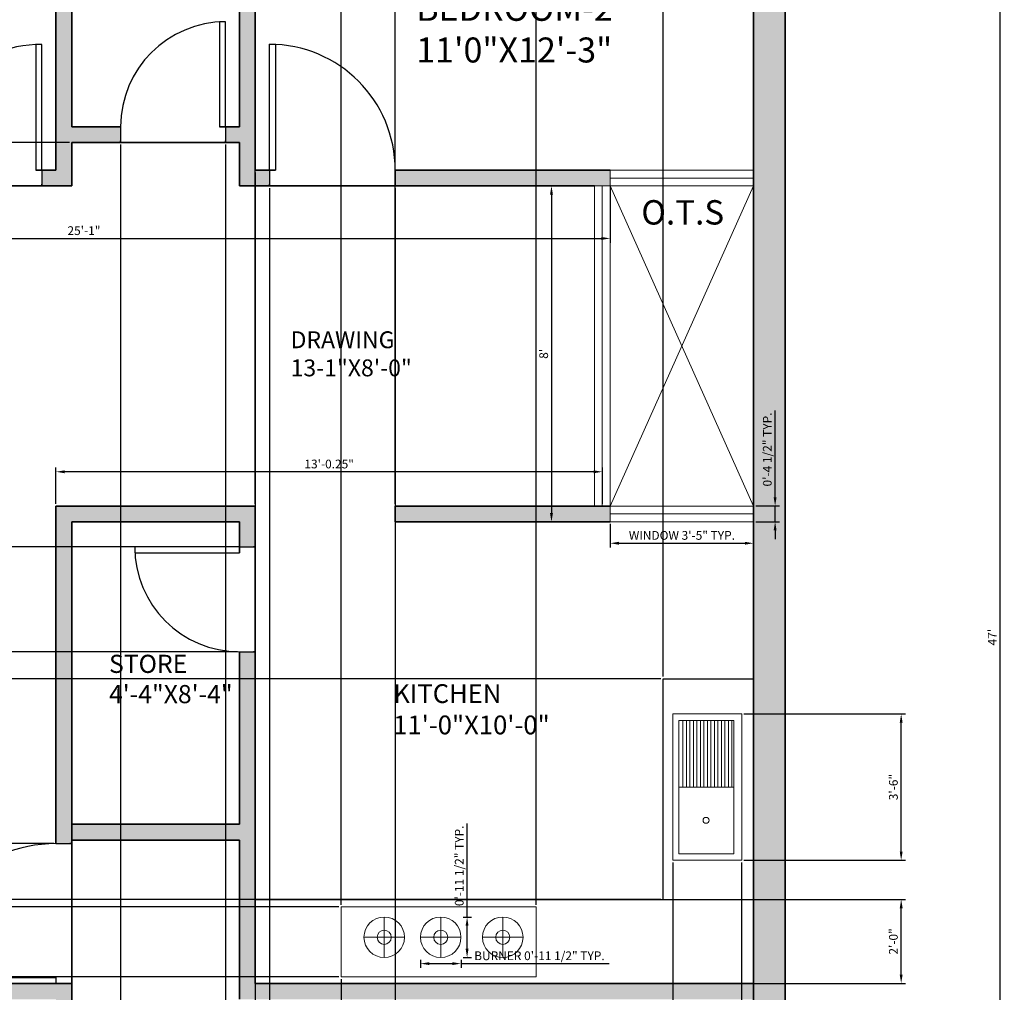
# Model space of a CAD drawing. Units: inches. Extents: x 2063 to 2524, y 2436 to 3097.
# Tile 3 of 4: x 2243 to 2524, y 2673 to 2951. Entities that reach past the tile are written whole.
import ezdxf

# ---------------------------------------------------------------- set-up
doc = ezdxf.new("R2010")
doc.units = ezdxf.units.IN
for name, color, linetype, lineweight in [('A-ANNO-DIMS', 2, 'Continuous', 18), ('A-AREA-IDEN', 7, 'Continuous', 18), ('A-DOOR', 4, 'Continuous', 25), ('A-EQPM', 8, 'Continuous', 18), ('A-FLOR-CASE', 8, 'Continuous', 25), ('A-FLOR-FIXT', 9, 'Continuous', 18), ('A-FLOR-FIXT-PATT', 9, 'Continuous', 13), ('A-FLOR-OPEN', 8, 'Continuous', 13), ('A-GLAZ', 5, 'Continuous', 18), ('A-WALL', 7, 'Continuous', 35)]:
    doc.layers.add(name, color=color, linetype=linetype, lineweight=lineweight)
doc.layers.add('A-WALL-PATT', color=251, linetype='Continuous', lineweight=13, true_color=0x636466)
doc.styles.get("Standard").update_dxf_attribs({"font": 'arial.ttf'})
doc.dimstyles.new('ISO-25', dxfattribs={"dimtxt": 2.5, "dimasz": 2.5, "dimexe": 1.25, "dimexo": 0.625, "dimtad": 1, "dimlunit": 3, "dimtxsty": 'Standard', "dimcen": 2.5, "dimadec": 0, "dimazin": 0, "dimtfac": 1, "dimtmove": 0, "dimatfit": 3, "dimfxl": 1, "dimarcsym": 0})

# ---------------------------------------------------------------- blocks, each defined once
blk = doc.blocks.new('*U3')
for p, q in [((0, 0), (0, -4)), ((-36, 0), (-36, -4))]:
    blk.add_line(p, q)
blk.add_lwpolyline([(0, 0), (0, 36), (-1.75, 36), (-1.75, 0)], close=True)
blk.add_arc((0, 0), 36, 90, 180)
blk = doc.blocks.new('*U4')
for p, q in [((-30, 0), (-30, -4)), ((0, 0), (0, -4))]:
    blk.add_line(p, q)
blk.add_lwpolyline([(0, 0), (0, 30), (-1.75, 30), (-1.75, 0)], close=True)
blk.add_arc((0, 0), 30, 90, 180)
blk = doc.blocks.new('*U2')
for p, q in [((0, 0), (0, -4)), ((36, 0), (36, -4))]:
    blk.add_line(p, q)
blk.add_lwpolyline([(0, 0), (0, 36), (1.75, 36), (1.75, 0)], close=True)
blk.add_arc((0, 0), 36, 0, 90)
blk = doc.blocks.new('*U6')
for p, q in [((-30, 0), (-30, -4)), ((0, 0), (0, -4))]:
    blk.add_line(p, q)
blk.add_lwpolyline([(0, 0), (0, 30), (-1.75, 30), (-1.75, 0)], close=True)
blk.add_arc((0, 0), 30, 90, 180)
blk = doc.blocks.new('*U5')
for p, q in [((0, 0), (0, -4)), ((40, 0), (40, -4))]:
    blk.add_line(p, q)
blk.add_lwpolyline([(0, 0), (0, 40), (1.75, 40), (1.75, 0)], close=True)
blk.add_arc((0, 0), 40, 0, 90)
blk = doc.blocks.new('*D11')
at = {"layer": 'A-ANNO-DIMS', "color": 0, "lineweight": -2, "transparency": 16777216}
for p, q in [((2110.76, 2902.49), (2110.76, 2886.87)), ((2411.76, 2902.49), (2411.76, 2886.87)), ((2113.26, 2888.12), (2409.26, 2888.12))]:
    blk.add_line(p, q, dxfattribs=at)
at = {"layer": 'A-ANNO-DIMS', "color": 0, "transparency": 16777216}
for points in [[(2113.26, 2888.53), (2113.26, 2887.7), (2110.76, 2888.12)], [(2409.26, 2888.53), (2409.26, 2887.7), (2411.76, 2888.12)]]:
    blk.add_solid(points, dxfattribs=at)
at = {"layer": 'Defpoints', "color": 0, "transparency": 16777216}
for p in [(2110.76, 2903.12), (2411.76, 2903.12), (2411.76, 2888.12)]:
    blk.add_point(p, dxfattribs=at)
at = {"layer": 'A-ANNO-DIMS', "color": 0, "transparency": 16777216, "insert": (2261.26, 2890.02), "char_height": 2.5, "attachment_point": 5}
blk.add_mtext('25\'-1"', dxfattribs=at)
blk = doc.blocks.new('*D12')
at = {"layer": 'A-ANNO-DIMS', "color": 0, "lineweight": -2, "transparency": 16777216}
for p, q in [((2406.64, 2903.12), (2393.71, 2903.12)), ((2394.96, 2900.62), (2394.96, 2809.62)), ((2406.64, 2807.12), (2393.71, 2807.12))]:
    blk.add_line(p, q, dxfattribs=at)
at = {"layer": 'A-ANNO-DIMS', "color": 0, "transparency": 16777216}
for points in [[(2394.54, 2900.62), (2395.38, 2900.62), (2394.96, 2903.12)], [(2394.54, 2809.62), (2395.38, 2809.62), (2394.96, 2807.12)]]:
    blk.add_solid(points, dxfattribs=at)
at = {"layer": 'Defpoints', "color": 0, "transparency": 16777216}
for p in [(2407.26, 2903.12), (2394.96, 2807.12), (2407.26, 2807.12)]:
    blk.add_point(p, dxfattribs=at)
at = {"layer": 'A-ANNO-DIMS', "color": 0, "transparency": 16777216, "insert": (2393.06, 2855.12), "char_height": 2.5, "attachment_point": 5, "rotation": 90}
blk.add_mtext("8'", dxfattribs=at)
blk = doc.blocks.new('*D13')
at = {"layer": 'A-ANNO-DIMS', "color": 0, "lineweight": -2, "transparency": 16777216}
for p, q in [((2253.26, 2812.24), (2253.26, 2822.65)), ((2407.01, 2821.4), (2255.76, 2821.4)), ((2409.51, 2812.24), (2409.51, 2822.65))]:
    blk.add_line(p, q, dxfattribs=at)
at = {"layer": 'A-ANNO-DIMS', "color": 0, "transparency": 16777216}
for points in [[(2255.76, 2821.81), (2255.76, 2820.98), (2253.26, 2821.4)], [(2407.01, 2821.81), (2407.01, 2820.98), (2409.51, 2821.4)]]:
    blk.add_solid(points, dxfattribs=at)
at = {"layer": 'Defpoints', "color": 0, "transparency": 16777216}
for p in [(2253.26, 2821.4), (2253.26, 2811.62), (2409.51, 2811.62)]:
    blk.add_point(p, dxfattribs=at)
at = {"layer": 'A-ANNO-DIMS', "color": 0, "transparency": 16777216, "insert": (2331.39, 2823.3), "char_height": 2.5, "attachment_point": 5}
blk.add_mtext('13\'-0.25"', dxfattribs=at)
blk = doc.blocks.new('*D15')
at = {"layer": 'A-ANNO-DIMS', "color": 0, "lineweight": -2, "transparency": 16777216}
for p, q in [((2462.39, 3056.12), (2524.46, 3056.12)), ((2523.21, 3053.62), (2523.21, 2494.62)), ((2462.39, 2492.12), (2524.46, 2492.12))]:
    blk.add_line(p, q, dxfattribs=at)
at = {"layer": 'A-ANNO-DIMS', "color": 0, "transparency": 16777216}
for points in [[(2522.79, 3053.62), (2523.62, 3053.62), (2523.21, 3056.12)], [(2522.79, 2494.62), (2523.62, 2494.62), (2523.21, 2492.12)]]:
    blk.add_solid(points, dxfattribs=at)
at = {"layer": 'Defpoints', "color": 0, "transparency": 16777216}
for p in [(2461.76, 3056.12), (2461.76, 2492.12), (2523.21, 2492.12)]:
    blk.add_point(p, dxfattribs=at)
at = {"layer": 'A-ANNO-DIMS', "color": 0, "transparency": 16777216, "insert": (2521.33, 2774.12), "char_height": 2.5, "attachment_point": 5, "rotation": 90}
blk.add_mtext("47'", dxfattribs=at)
blk = doc.blocks.new('COOKTOP-BURNER')
for p, q in [((5.79, 11.58), (5.79, 0)), ((5.79, 5.79), (0, 5.79)), ((5.79, 0), (5.79, 5.79)), ((5.79, 5.79), (11.58, 5.79)), ((11.58, 5.79), (5.79, 5.79))]:
    blk.add_line(p, q)
for radius in [5.79, 2.02]:
    blk.add_circle((5.79, 5.79), radius)
blk = doc.blocks.new('WIN-OTS-41IN')
for p, q in [((0, 4.5), (41, 4.5)), ((0, 2.25), (41, 2.25)), ((0, 0), (41, 0))]:
    blk.add_line(p, q)
blk = doc.blocks.new('*D22')
at = {"layer": 'A-ANNO-DIMS', "color": 0, "lineweight": -2, "transparency": 16777216}
for p, q in [((2357.51, 2681.89), (2357.51, 2679.53)), ((2360.01, 2680.78), (2366.59, 2680.78)), ((2369.09, 2681.89), (2369.09, 2679.53)), ((2369.09, 2680.78), (2411.45, 2680.78))]:
    blk.add_line(p, q, dxfattribs=at)
at = {"layer": 'A-ANNO-DIMS', "color": 0, "transparency": 16777216}
for points in [[(2360.01, 2681.2), (2360.01, 2680.37), (2357.51, 2680.78)], [(2366.59, 2681.2), (2366.59, 2680.37), (2369.09, 2680.78)]]:
    blk.add_solid(points, dxfattribs=at)
at = {"layer": 'Defpoints', "color": 0, "transparency": 16777216}
for p in [(2357.51, 2682.52), (2369.09, 2682.52), (2369.09, 2680.78)]:
    blk.add_point(p, dxfattribs=at)
at = {"layer": 'A-ANNO-DIMS', "color": 0, "transparency": 16777216, "insert": (2391.52, 2682.7), "char_height": 2.5, "attachment_point": 5}
blk.add_mtext('BURNER 0\'-11 1/2" TYP.', dxfattribs=at)
blk = doc.blocks.new('*D23')
at = {"layer": 'A-ANNO-DIMS', "color": 0, "lineweight": -2, "transparency": 16777216}
for p, q in [((2370.83, 2694.1), (2370.83, 2720.86)), ((2369.71, 2694.1), (2372.08, 2694.1)), ((2370.83, 2685.02), (2370.83, 2691.6)), ((2369.71, 2682.52), (2372.08, 2682.52))]:
    blk.add_line(p, q, dxfattribs=at)
at = {"layer": 'A-ANNO-DIMS', "color": 0, "transparency": 16777216}
for points in [[(2370.41, 2691.6), (2371.24, 2691.6), (2370.83, 2694.1)], [(2370.41, 2685.02), (2371.24, 2685.02), (2370.83, 2682.52)]]:
    blk.add_solid(points, dxfattribs=at)
at = {"layer": 'Defpoints', "color": 0, "transparency": 16777216}
for p in [(2369.09, 2694.1), (2370.83, 2694.1), (2369.09, 2682.52)]:
    blk.add_point(p, dxfattribs=at)
at = {"layer": 'A-ANNO-DIMS', "color": 0, "transparency": 16777216, "insert": (2368.91, 2708.73), "char_height": 2.5, "attachment_point": 5, "rotation": 90}
blk.add_mtext('0\'-11 1/2" TYP.', dxfattribs=at)
blk = doc.blocks.new('*D26')
at = {"layer": 'A-ANNO-DIMS', "color": 0, "lineweight": -2, "transparency": 16777216}
for p, q in [((2411.76, 2806.49), (2411.76, 2799.72)), ((2452.76, 2806.49), (2452.76, 2799.72)), ((2414.26, 2800.97), (2450.26, 2800.97))]:
    blk.add_line(p, q, dxfattribs=at)
at = {"layer": 'A-ANNO-DIMS', "color": 0, "transparency": 16777216}
for points in [[(2414.26, 2801.38), (2414.26, 2800.55), (2411.76, 2800.97)], [(2450.26, 2801.38), (2450.26, 2800.55), (2452.76, 2800.97)]]:
    blk.add_solid(points, dxfattribs=at)
at = {"layer": 'Defpoints', "color": 0, "transparency": 16777216}
for p in [(2411.76, 2807.12), (2452.76, 2807.12), (2452.76, 2800.97)]:
    blk.add_point(p, dxfattribs=at)
at = {"layer": 'A-ANNO-DIMS', "color": 0, "transparency": 16777216, "insert": (2432.26, 2802.89), "char_height": 2.5, "attachment_point": 5}
blk.add_mtext('WINDOW 3\'-5" TYP.', dxfattribs=at)
blk = doc.blocks.new('*D27')
at = {"layer": 'A-ANNO-DIMS', "color": 0, "lineweight": -2, "transparency": 16777216}
for p, q in [((2458.91, 2814.12), (2458.91, 2838.93)), ((2453.39, 2811.62), (2460.16, 2811.62)), ((2458.91, 2807.12), (2458.91, 2811.62)), ((2453.39, 2807.12), (2460.16, 2807.12)), ((2458.91, 2804.62), (2458.91, 2802.12))]:
    blk.add_line(p, q, dxfattribs=at)
at = {"layer": 'A-ANNO-DIMS', "color": 0, "transparency": 16777216}
for points in [[(2458.5, 2814.12), (2459.33, 2814.12), (2458.91, 2811.62)], [(2458.5, 2804.62), (2459.33, 2804.62), (2458.91, 2807.12)]]:
    blk.add_solid(points, dxfattribs=at)
at = {"layer": 'Defpoints', "color": 0, "transparency": 16777216}
for p in [(2452.76, 2811.62), (2458.91, 2811.62), (2452.76, 2807.12)]:
    blk.add_point(p, dxfattribs=at)
at = {"layer": 'A-ANNO-DIMS', "color": 0, "transparency": 16777216, "insert": (2457, 2827.77), "char_height": 2.5, "attachment_point": 5, "rotation": 90}
blk.add_mtext('0\'-4 1/2" TYP.', dxfattribs=at)
blk = doc.blocks.new('*D34')
at = {"layer": 'A-ANNO-DIMS', "color": 0, "lineweight": -2, "transparency": 16777216}
for p, q in [((2271.76, 2914.94), (2271.76, 2457.67)), ((2301.76, 2914.94), (2301.76, 2457.67)), ((2274.26, 2458.92), (2299.26, 2458.92))]:
    blk.add_line(p, q, dxfattribs=at)
at = {"layer": 'A-ANNO-DIMS', "color": 0, "transparency": 16777216}
for points in [[(2274.26, 2459.33), (2274.26, 2458.5), (2271.76, 2458.92)], [(2299.26, 2459.33), (2299.26, 2458.5), (2301.76, 2458.92)]]:
    blk.add_solid(points, dxfattribs=at)
at = {"layer": 'Defpoints', "color": 0, "transparency": 16777216}
for p in [(2271.76, 2915.57), (2301.76, 2915.57), (2301.76, 2458.92)]:
    blk.add_point(p, dxfattribs=at)
at = {"layer": 'A-ANNO-DIMS', "color": 0, "transparency": 16777216, "insert": (2286.76, 2460.82), "char_height": 2.5, "attachment_point": 5}
blk.add_mtext('2\'-6"', dxfattribs=at)
blk = doc.blocks.new('*D35')
at = {"layer": 'A-ANNO-DIMS', "color": 0, "lineweight": -2, "transparency": 16777216}
for p, q in [((2068.56, 2915.57), (2068.56, 2931.55)), ((2257.14, 2915.57), (2067.31, 2915.57)), ((2068.56, 2905.62), (2068.56, 2913.07)), ((2257.14, 2903.12), (2067.31, 2903.12))]:
    blk.add_line(p, q, dxfattribs=at)
at = {"layer": 'A-ANNO-DIMS', "color": 0, "transparency": 16777216}
for points in [[(2068.15, 2913.07), (2068.98, 2913.07), (2068.56, 2915.57)], [(2068.15, 2905.62), (2068.98, 2905.62), (2068.56, 2903.12)]]:
    blk.add_solid(points, dxfattribs=at)
at = {"layer": 'Defpoints', "color": 0, "transparency": 16777216}
for p in [(2068.56, 2915.57), (2257.76, 2915.57), (2257.76, 2903.12)]:
    blk.add_point(p, dxfattribs=at)
at = {"layer": 'A-ANNO-DIMS', "color": 0, "transparency": 16777216, "insert": (2066.65, 2924.81), "char_height": 2.5, "attachment_point": 5, "rotation": 90}
blk.add_mtext('1\'-0 1/2"', dxfattribs=at)
blk = doc.blocks.new('*D36')
at = {"layer": 'A-ANNO-DIMS', "color": 0, "lineweight": -2, "transparency": 16777216}
for p, q in [((2314.3, 2902.49), (2314.3, 2457.67)), ((2350.3, 2902.49), (2350.3, 2457.67)), ((2316.8, 2458.92), (2347.8, 2458.92))]:
    blk.add_line(p, q, dxfattribs=at)
at = {"layer": 'A-ANNO-DIMS', "color": 0, "transparency": 16777216}
for points in [[(2316.8, 2459.33), (2316.8, 2458.5), (2314.3, 2458.92)], [(2347.8, 2459.33), (2347.8, 2458.5), (2350.3, 2458.92)]]:
    blk.add_solid(points, dxfattribs=at)
at = {"layer": 'Defpoints', "color": 0, "transparency": 16777216}
for p in [(2314.3, 2903.12), (2350.3, 2903.12), (2350.3, 2458.92)]:
    blk.add_point(p, dxfattribs=at)
at = {"layer": 'A-ANNO-DIMS', "color": 0, "transparency": 16777216, "insert": (2332.3, 2460.82), "char_height": 2.5, "attachment_point": 5}
blk.add_mtext('3\'-0"', dxfattribs=at)
blk = doc.blocks.new('*D38')
at = {"layer": 'A-ANNO-DIMS', "color": 0, "lineweight": -2, "transparency": 16777216}
for p, q in [((2310.26, 2812.24), (2310.26, 3090.57)), ((2312.76, 3089.32), (2347.8, 3089.32)), ((2350.3, 2812.24), (2350.3, 3090.57))]:
    blk.add_line(p, q, dxfattribs=at)
at = {"layer": 'A-ANNO-DIMS', "color": 0, "transparency": 16777216}
for points in [[(2312.76, 3089.73), (2312.76, 3088.9), (2310.26, 3089.32)], [(2347.8, 3089.73), (2347.8, 3088.9), (2350.3, 3089.32)]]:
    blk.add_solid(points, dxfattribs=at)
at = {"layer": 'Defpoints', "color": 0, "transparency": 16777216}
for p in [(2350.3, 3089.32), (2310.26, 2811.62), (2350.3, 2811.62)]:
    blk.add_point(p, dxfattribs=at)
at = {"layer": 'A-ANNO-DIMS', "color": 0, "transparency": 16777216, "insert": (2330.28, 3091.22), "char_height": 2.5, "attachment_point": 5}
blk.add_mtext('3\'-4"', dxfattribs=at)
blk = doc.blocks.new('*D39')
at = {"layer": 'A-ANNO-DIMS', "color": 0, "lineweight": -2, "transparency": 16777216}
for p, q in [((2426.9, 2762.84), (2426.9, 3090.57)), ((2429.4, 3089.32), (2450.26, 3089.32)), ((2452.76, 2762.84), (2452.76, 3090.57))]:
    blk.add_line(p, q, dxfattribs=at)
at = {"layer": 'A-ANNO-DIMS', "color": 0, "transparency": 16777216}
for points in [[(2429.4, 3089.73), (2429.4, 3088.9), (2426.9, 3089.32)], [(2450.26, 3089.73), (2450.26, 3088.9), (2452.76, 3089.32)]]:
    blk.add_solid(points, dxfattribs=at)
at = {"layer": 'Defpoints', "color": 0, "transparency": 16777216}
for p in [(2452.76, 3089.32), (2426.9, 2762.21), (2452.76, 2762.21)]:
    blk.add_point(p, dxfattribs=at)
at = {"layer": 'A-ANNO-DIMS', "color": 0, "transparency": 16777216, "insert": (2439.83, 3091.2), "char_height": 2.5, "attachment_point": 5}
blk.add_mtext('2\'-2"', dxfattribs=at)
blk = doc.blocks.new('*D40')
at = {"layer": 'A-ANNO-DIMS', "color": 0, "lineweight": -2, "transparency": 16777216}
for p, q in [((2310.89, 2699.12), (2496.21, 2699.12)), ((2494.96, 2677.62), (2494.96, 2696.62)), ((2310.89, 2675.12), (2496.21, 2675.12))]:
    blk.add_line(p, q, dxfattribs=at)
at = {"layer": 'A-ANNO-DIMS', "color": 0, "transparency": 16777216}
for points in [[(2494.55, 2696.62), (2495.38, 2696.62), (2494.96, 2699.12)], [(2494.55, 2677.62), (2495.38, 2677.62), (2494.96, 2675.12)]]:
    blk.add_solid(points, dxfattribs=at)
at = {"layer": 'Defpoints', "color": 0, "transparency": 16777216}
for p in [(2310.26, 2699.12), (2494.96, 2699.12), (2310.26, 2675.12)]:
    blk.add_point(p, dxfattribs=at)
at = {"layer": 'A-ANNO-DIMS', "color": 0, "transparency": 16777216, "insert": (2493.06, 2687.12), "char_height": 2.5, "attachment_point": 5, "rotation": 90}
blk.add_mtext('2\'-0"', dxfattribs=at)
blk = doc.blocks.new('*D41')
at = {"layer": 'A-ANNO-DIMS', "color": 0, "lineweight": -2, "transparency": 16777216}
for p, q in [((2305.15, 2799.95), (2067.31, 2799.95)), ((2068.56, 2772.45), (2068.56, 2797.45)), ((2305.14, 2769.95), (2067.31, 2769.95))]:
    blk.add_line(p, q, dxfattribs=at)
at = {"layer": 'A-ANNO-DIMS', "color": 0, "transparency": 16777216}
for points in [[(2068.15, 2797.45), (2068.98, 2797.45), (2068.56, 2799.95)], [(2068.15, 2772.45), (2068.98, 2772.45), (2068.56, 2769.95)]]:
    blk.add_solid(points, dxfattribs=at)
at = {"layer": 'Defpoints', "color": 0, "transparency": 16777216}
for p in [(2068.56, 2799.95), (2305.78, 2799.95), (2305.76, 2769.95)]:
    blk.add_point(p, dxfattribs=at)
at = {"layer": 'A-ANNO-DIMS', "color": 0, "transparency": 16777216, "insert": (2066.66, 2784.95), "char_height": 2.5, "attachment_point": 5, "rotation": 90}
blk.add_mtext('2\'-6"', dxfattribs=at)
blk = doc.blocks.new('*D42')
at = {"layer": 'A-ANNO-DIMS', "color": 0, "lineweight": -2, "transparency": 16777216}
for p, q in [((2426.27, 2762.21), (2067.31, 2762.21)), ((2068.56, 2701.62), (2068.56, 2759.71)), ((2426.27, 2699.12), (2067.31, 2699.12))]:
    blk.add_line(p, q, dxfattribs=at)
at = {"layer": 'A-ANNO-DIMS', "color": 0, "transparency": 16777216}
for points in [[(2068.15, 2759.71), (2068.98, 2759.71), (2068.56, 2762.21)], [(2068.15, 2701.62), (2068.98, 2701.62), (2068.56, 2699.12)]]:
    blk.add_solid(points, dxfattribs=at)
at = {"layer": 'Defpoints', "color": 0, "transparency": 16777216}
for p in [(2068.56, 2762.21), (2426.9, 2762.21), (2426.9, 2699.12)]:
    blk.add_point(p, dxfattribs=at)
at = {"layer": 'A-ANNO-DIMS', "color": 0, "transparency": 16777216, "insert": (2066.66, 2730.67), "char_height": 2.5, "attachment_point": 5, "rotation": 90}
blk.add_mtext('5\'-3"', dxfattribs=at)
blk = doc.blocks.new('*D43')
at = {"layer": 'A-ANNO-DIMS', "color": 0, "lineweight": -2, "transparency": 16777216}
for p, q in [((2429.67, 2709.7), (2429.67, 2457.67)), ((2449.35, 2709.7), (2449.35, 2457.67)), ((2432.17, 2458.92), (2446.85, 2458.92))]:
    blk.add_line(p, q, dxfattribs=at)
at = {"layer": 'A-ANNO-DIMS', "color": 0, "transparency": 16777216}
for points in [[(2432.17, 2459.33), (2432.17, 2458.5), (2429.67, 2458.92)], [(2446.85, 2459.33), (2446.85, 2458.5), (2449.35, 2458.92)]]:
    blk.add_solid(points, dxfattribs=at)
at = {"layer": 'Defpoints', "color": 0, "transparency": 16777216}
for p in [(2429.67, 2710.33), (2449.35, 2710.33), (2449.35, 2458.92)]:
    blk.add_point(p, dxfattribs=at)
at = {"layer": 'A-ANNO-DIMS', "color": 0, "transparency": 16777216, "insert": (2439.51, 2460.84), "char_height": 2.5, "attachment_point": 5}
blk.add_mtext('1\'-7 1/2"', dxfattribs=at)
blk = doc.blocks.new('*D44')
at = {"layer": 'A-ANNO-DIMS', "color": 0, "lineweight": -2, "transparency": 16777216}
for p, q in [((2449.98, 2752.17), (2496.21, 2752.17)), ((2494.96, 2712.83), (2494.96, 2749.67)), ((2449.98, 2710.33), (2496.21, 2710.33))]:
    blk.add_line(p, q, dxfattribs=at)
at = {"layer": 'A-ANNO-DIMS', "color": 0, "transparency": 16777216}
for points in [[(2494.55, 2749.67), (2495.38, 2749.67), (2494.96, 2752.17)], [(2494.55, 2712.83), (2495.38, 2712.83), (2494.96, 2710.33)]]:
    blk.add_solid(points, dxfattribs=at)
at = {"layer": 'Defpoints', "color": 0, "transparency": 16777216}
for p in [(2449.35, 2752.17), (2494.96, 2752.17), (2449.35, 2710.33)]:
    blk.add_point(p, dxfattribs=at)
at = {"layer": 'A-ANNO-DIMS', "color": 0, "transparency": 16777216, "insert": (2493.06, 2731.25), "char_height": 2.5, "attachment_point": 5, "rotation": 90}
blk.add_mtext('3\'-6"', dxfattribs=at)
blk = doc.blocks.new('*D45')
at = {"layer": 'A-ANNO-DIMS', "color": 0, "lineweight": -2, "transparency": 16777216}
for p, q in [((2252.63, 2715.09), (2067.31, 2715.09)), ((2068.56, 2677.62), (2068.56, 2712.59)), ((2252.64, 2675.12), (2067.31, 2675.12))]:
    blk.add_line(p, q, dxfattribs=at)
at = {"layer": 'A-ANNO-DIMS', "color": 0, "transparency": 16777216}
for points in [[(2068.15, 2712.59), (2068.98, 2712.59), (2068.56, 2715.09)], [(2068.15, 2677.62), (2068.98, 2677.62), (2068.56, 2675.12)]]:
    blk.add_solid(points, dxfattribs=at)
at = {"layer": 'Defpoints', "color": 0, "transparency": 16777216}
for p in [(2068.56, 2715.09), (2253.26, 2715.09), (2253.26, 2675.12)]:
    blk.add_point(p, dxfattribs=at)
at = {"layer": 'A-ANNO-DIMS', "color": 0, "transparency": 16777216, "insert": (2066.66, 2695.1), "char_height": 2.5, "attachment_point": 5, "rotation": 90}
blk.add_mtext('3\'-4"', dxfattribs=at)
blk = doc.blocks.new('*D48')
at = {"layer": 'A-ANNO-DIMS', "color": 0, "lineweight": -2, "transparency": 16777216}
for p, q in [((2310.26, 2906.99), (2310.26, 2457.67)), ((2314.3, 2902.49), (2314.3, 2457.67)), ((2307.76, 2458.92), (2305.26, 2458.92)), ((2310.26, 2458.92), (2314.3, 2458.92)), ((2316.8, 2458.92), (2327.2, 2458.92))]:
    blk.add_line(p, q, dxfattribs=at)
at = {"layer": 'A-ANNO-DIMS', "color": 0, "transparency": 16777216}
for points in [[(2307.76, 2459.33), (2307.76, 2458.5), (2310.26, 2458.92)], [(2316.8, 2459.33), (2316.8, 2458.5), (2314.3, 2458.92)]]:
    blk.add_solid(points, dxfattribs=at)
at = {"layer": 'Defpoints', "color": 0, "transparency": 16777216}
for p in [(2310.26, 2907.62), (2314.3, 2903.12), (2314.3, 2458.92)]:
    blk.add_point(p, dxfattribs=at)
at = {"layer": 'A-ANNO-DIMS', "color": 0, "transparency": 16777216, "insert": (2323.25, 2460.82), "char_height": 2.5, "attachment_point": 5}
blk.add_mtext('0\'-4"', dxfattribs=at)
blk = doc.blocks.new('*D49')
at = {"layer": 'A-ANNO-DIMS', "color": 0, "lineweight": -2, "transparency": 16777216}
for p, q in [((2334.8, 2697.62), (2334.8, 3090.57)), ((2337.3, 3089.32), (2388.07, 3089.32)), ((2390.57, 2697.62), (2390.57, 3090.57))]:
    blk.add_line(p, q, dxfattribs=at)
at = {"layer": 'A-ANNO-DIMS', "color": 0, "transparency": 16777216}
for points in [[(2337.3, 3089.73), (2337.3, 3088.9), (2334.8, 3089.32)], [(2388.07, 3089.73), (2388.07, 3088.9), (2390.57, 3089.32)]]:
    blk.add_solid(points, dxfattribs=at)
at = {"layer": 'Defpoints', "color": 0, "transparency": 16777216}
for p in [(2390.57, 3089.32), (2334.8, 2696.99), (2390.57, 2696.99)]:
    blk.add_point(p, dxfattribs=at)
at = {"layer": 'A-ANNO-DIMS', "color": 0, "transparency": 16777216, "insert": (2362.68, 3091.22), "char_height": 2.5, "attachment_point": 5}
blk.add_mtext('4\'-8"', dxfattribs=at)
blk = doc.blocks.new('*D50')
at = {"layer": 'A-ANNO-DIMS', "color": 0, "lineweight": -2, "transparency": 16777216}
for p, q in [((2334.17, 2696.99), (2067.31, 2696.99)), ((2068.56, 2679.49), (2068.56, 2694.49)), ((2334.17, 2676.99), (2067.31, 2676.99))]:
    blk.add_line(p, q, dxfattribs=at)
at = {"layer": 'A-ANNO-DIMS', "color": 0, "transparency": 16777216}
for points in [[(2068.15, 2694.49), (2068.98, 2694.49), (2068.56, 2696.99)], [(2068.15, 2679.49), (2068.98, 2679.49), (2068.56, 2676.99)]]:
    blk.add_solid(points, dxfattribs=at)
at = {"layer": 'Defpoints', "color": 0, "transparency": 16777216}
for p in [(2068.56, 2696.99), (2334.8, 2696.99), (2334.8, 2676.99)]:
    blk.add_point(p, dxfattribs=at)
at = {"layer": 'A-ANNO-DIMS', "color": 0, "transparency": 16777216, "insert": (2066.66, 2686.99), "char_height": 2.5, "attachment_point": 5, "rotation": 90}
blk.add_mtext('1\'-8"', dxfattribs=at)
blk = doc.blocks.new('*D51')
at = {"layer": 'A-ANNO-DIMS', "color": 0, "lineweight": -2, "transparency": 16777216}
for p, q in [((2334.8, 2676.36), (2334.8, 2457.67)), ((2310.26, 2674.49), (2310.26, 2457.67)), ((2312.76, 2458.92), (2332.3, 2458.92))]:
    blk.add_line(p, q, dxfattribs=at)
at = {"layer": 'A-ANNO-DIMS', "color": 0, "transparency": 16777216}
for points in [[(2312.76, 2459.33), (2312.76, 2458.5), (2310.26, 2458.92)], [(2332.3, 2459.33), (2332.3, 2458.5), (2334.8, 2458.92)]]:
    blk.add_solid(points, dxfattribs=at)
at = {"layer": 'Defpoints', "color": 0, "transparency": 16777216}
for p in [(2310.26, 2675.12), (2334.8, 2676.99), (2334.8, 2458.92)]:
    blk.add_point(p, dxfattribs=at)
at = {"layer": 'A-ANNO-DIMS', "color": 0, "transparency": 16777216, "insert": (2322.53, 2460.84), "char_height": 2.5, "attachment_point": 5}
blk.add_mtext('2\'-0 1/2"', dxfattribs=at)

msp = doc.modelspace()

# ---------------------------------------------------------------- hatches: boundary and pattern name
at = {"layer": 'A-FLOR-FIXT-PATT'}
h = msp.add_hatch(dxfattribs=at)
h.set_pattern_fill('ANSI31', color=256, scale=0.3149013, angle=45, style=0)
h.paths.add_polyline_path([(2432.04, 2731.223), (2447.04, 2731.223), (2447.04, 2750.267), (2432.04, 2750.267)])
at = {"layer": 'A-WALL-PATT'}
h = msp.add_hatch(color=256, dxfattribs=at)
h.dxf.hatch_style = 1
h.paths.add_polyline_path([(2110.763, 2670.618), (2110.763, 2676.643), (2110.763, 3047.118), (2452.763, 3047.118), (2452.763, 2501.118), (2200.478, 2501.118), (2200.478, 2492.118), (2461.763, 2492.118), (2461.763, 3056.118), (2101.763, 3056.118), (2101.763, 2492.118), (2149.478, 2492.118), (2149.478, 2496.618), (2149.478, 2501.118), (2110.763, 2501.118)])
h.paths.add_polyline_path([(2257.763, 2675.118), (2257.255, 2675.091), (2253.255, 2675.091), (2213.255, 2675.091), (2151.474, 2675.107), (2151.474, 2674.543), (2151.474, 2670.618), (2253.263, 2670.618), (2253.263, 2501.118), (2257.763, 2501.118)], flags=17)
h.paths.add_polyline_path([(2310.263, 3006.972), (2305.763, 3006.972), (2305.763, 2920.067), (2301.763, 2920.067), (2301.759, 2920.067), (2301.759, 2920.063), (2301.759, 2916.063), (2301.759, 2915.567), (2305.763, 2915.567), (2305.763, 2903.118), (2314.3, 2903.118), (2314.3, 2903.618), (2314.3, 2907.618), (2310.263, 2907.618)], flags=17)
h.paths.add_polyline_path([(2257.763, 3006.972), (2253.263, 3006.972), (2253.263, 2907.618), (2249.263, 2907.618), (2249.258, 2907.618), (2249.258, 2907.597), (2249.258, 2903.597), (2249.258, 2903.118), (2257.763, 2903.118), (2257.763, 2915.567), (2271.759, 2915.567), (2271.759, 2916.063), (2271.759, 2920.067), (2257.763, 2920.067)], flags=17)
h.paths.add_polyline_path([(2213.258, 2907.618), (2110.763, 2907.618), (2110.763, 2903.118), (2213.258, 2903.118), (2213.258, 2903.597)], flags=17)
h.paths.add_polyline_path([(2411.763, 2907.618), (2350.3, 2907.618), (2350.3, 2903.618), (2350.3, 2903.118), (2407.264, 2903.118), (2411.763, 2903.118)], flags=17)
h.paths.add_polyline_path([(2260.327, 2964.034), (2307.905, 2964.034), (2307.905, 2989.359), (2260.327, 2989.359)], flags=25)
h = msp.add_hatch(color=256, dxfattribs=at)
h.dxf.hatch_style = 1
h.paths.add_polyline_path([(2310.263, 2811.618), (2305.763, 2811.618), (2253.263, 2811.618), (2253.263, 2716.118), (2253.255, 2715.091), (2257.255, 2715.091), (2257.763, 2715.091), (2257.763, 2720.618), (2257.763, 2807.118), (2305.763, 2807.118), (2305.763, 2799.95), (2305.776, 2799.95), (2309.776, 2799.95), (2310.263, 2799.95)])
h.paths.add_polyline_path([(2310.263, 2769.95), (2309.776, 2769.95), (2305.763, 2769.95), (2305.763, 2720.618), (2257.763, 2720.618), (2257.763, 2716.118), (2305.763, 2716.118), (2305.763, 2670.618), (2310.263, 2670.618), (2452.763, 2670.618), (2452.763, 2675.118), (2426.899, 2675.118), (2310.263, 2675.118)])
h = msp.add_hatch(color=256, dxfattribs=at)
h.dxf.hatch_style = 1
h.paths.add_polyline_path([(2411.763, 2809.368), (2411.763, 2811.618), (2407.264, 2811.618), (2350.3, 2811.618), (2350.3, 2807.118), (2411.763, 2807.118)])

# ---------------------------------------------------------------- linework, layer by layer
at = {"layer": 'A-EQPM'}
msp.add_lwpolyline([(2334.798, 2696.991), (2390.571, 2696.991), (2390.571, 2676.988), (2334.798, 2676.988)], close=True, dxfattribs=at)
at = {"layer": 'A-FLOR-CASE'}
for p, q in [((2426.899, 2699.118), (2426.899, 2762.214)), ((2426.899, 2762.214), (2452.763, 2762.214)), ((2310.263, 2675.118), (2310.263, 2699.118)), ((2310.263, 2699.118), (2426.899, 2699.118))]:
    msp.add_line(p, q, dxfattribs=at)
at = {"layer": 'A-FLOR-FIXT'}
msp.add_line((2447.154, 2731.223), (2431.371, 2731.223), dxfattribs=at)
for points in [[(2429.674, 2752.175), (2449.352, 2752.175), (2449.352, 2710.326), (2429.674, 2710.326)], [(2431.371, 2750.267), (2447.154, 2750.267), (2447.154, 2712.179), (2431.371, 2712.179)]]:
    msp.add_lwpolyline(points, close=True, dxfattribs=at)
msp.add_circle((2439.167, 2721.751), 0.85, dxfattribs=at)
at = {"layer": 'A-FLOR-OPEN'}
for p, q in [((2452.763, 2903.118), (2411.763, 2811.618)), ((2411.763, 2903.118), (2452.763, 2811.618))]:
    msp.add_line(p, q, dxfattribs=at)
at = {"layer": 'A-GLAZ'}
for p, q in [((2411.763, 2903.118), (2411.763, 2907.618)), ((2407.264, 2903.118), (2407.264, 2811.618)), ((2411.763, 2903.118), (2407.264, 2903.118)), ((2409.502, 2903.118), (2409.502, 2811.618)), ((2411.763, 2903.118), (2411.763, 2811.618)), ((2407.264, 2811.618), (2411.763, 2811.618)), ((2411.763, 2811.618), (2411.763, 2807.118)), ((2411.763, 2807.118), (2411.763, 2809.368))]:
    msp.add_line(p, q, dxfattribs=at)
at = {"layer": 'A-WALL'}
for p, q in [((2461.763, 3056.118), (2461.763, 2492.118)), ((2452.763, 3047.118), (2452.763, 2501.118)), ((2253.263, 2907.618), (2253.263, 3006.972)), ((2257.763, 2920.067), (2257.763, 3006.972)), ((2305.763, 3006.972), (2305.763, 2920.067)), ((2310.263, 3006.972), (2310.263, 2907.618)), ((2257.763, 2920.067), (2271.759, 2920.067)), ((2300.009, 2920.067), (2305.763, 2920.067)), ((2305.763, 2920.067), (2301.763, 2920.067)), ((2257.763, 2915.567), (2305.763, 2915.567)), ((2257.763, 2903.118), (2257.763, 2915.567)), ((2271.759, 2916.063), (2271.759, 2915.567)), ((2301.759, 2916.063), (2301.759, 2915.567)), ((2305.763, 2915.567), (2305.763, 2903.118)), ((2247.508, 2907.618), (2253.263, 2907.618)), ((2253.263, 2907.618), (2249.263, 2907.618)), ((2310.263, 2907.618), (2316.05, 2907.618)), ((2350.3, 2907.618), (2411.763, 2907.618)), ((2110.763, 2903.118), (2257.763, 2903.118)), ((2249.258, 2903.597), (2249.258, 2903.118)), ((2305.763, 2903.118), (2407.264, 2903.118)), ((2314.3, 2903.618), (2314.3, 2903.118)), ((2350.3, 2903.618), (2350.3, 2903.118)), ((2305.763, 2811.618), (2253.263, 2811.618)), ((2253.263, 2811.618), (2253.263, 2716.118)), ((2305.763, 2811.618), (2310.263, 2811.618)), ((2310.263, 2811.618), (2310.263, 2675.118)), ((2350.3, 2811.618), (2350.3, 2807.118)), ((2350.3, 2811.618), (2411.763, 2811.618)), ((2305.763, 2807.118), (2257.763, 2807.118)), ((2257.763, 2720.618), (2257.763, 2807.118)), ((2305.763, 2807.118), (2305.763, 2798.2)), ((2350.3, 2807.118), (2411.763, 2807.118)), ((2309.776, 2799.95), (2310.263, 2799.95)), ((2305.763, 2769.95), (2305.763, 2720.618)), ((2309.776, 2769.95), (2310.263, 2769.95)), ((2257.763, 2720.618), (2305.763, 2720.618)), ((2257.763, 2675.118), (2257.763, 2720.618)), ((2253.263, 2716.118), (2253.255, 2715.091)), ((2257.255, 2715.091), (2257.763, 2715.091)), ((2257.763, 2716.118), (2305.763, 2716.118)), ((2305.763, 2716.118), (2305.763, 2670.618)), ((2257.763, 2675.118), (2110.763, 2675.118)), ((2253.263, 2675.091), (2253.263, 2675.118)), ((2257.255, 2675.091), (2257.763, 2675.118)), ((2257.763, 2501.118), (2257.763, 2675.118)), ((2452.763, 2675.118), (2310.263, 2675.118)), ((2452.763, 2675.118), (2426.899, 2675.118))]:
    msp.add_line(p, q, dxfattribs=at)

# ---------------------------------------------------------------- block references
at = {"layer": 'A-DOOR'}
for name, p in [('*U4', (2301.759, 2920.063)), ('*U3', (2249.258, 2907.597)), ('*U2', (2314.3, 2907.618))]:
    msp.add_blockref(name, p, dxfattribs=at)
at = {"layer": 'A-DOOR', "rotation": 90}
for name, p in [('*U6', (2305.776, 2799.95)), ('*U5', (2253.255, 2675.091))]:
    msp.add_blockref(name, p, dxfattribs=at)
at = {"layer": 'A-EQPM'}
for p in [(2341.345, 2682.519), (2357.507, 2682.519), (2375.245, 2682.519)]:
    msp.add_blockref('COOKTOP-BURNER', p, dxfattribs=at)
at = {"layer": 'A-GLAZ'}
for p in [(2411.763, 2903.118), (2411.763, 2807.118)]:
    msp.add_blockref('WIN-OTS-41IN', p, dxfattribs=at)

# ---------------------------------------------------------------- texts
at = {"layer": 'A-AREA-IDEN', "attachment_point": 1}
for s, width, gutter_width, heights, insert, char_height in [('BEDROOM-2\\P11\'0"X12\'-3"', 18.93706, 35.717, [0], (2356.274, 2957.479), 7.1434), ('O.T.S\\P\\P ', 46.75319, 34.807, [30.29], (2420.653, 2899.055), 6.9614), ('DRAWING\\P13-1"X8\'-0"', 4.54791, 24.123, [0], (2320.364, 2861.56), 4.82454), ('STORE\\P4\'-4"X8\'-4"', 52.10892, 25.944, [0], (2268.441, 2769.081), 5.18882), ('\\pxt2;KITCHEN\\P11\'-0"X10\'-0"', 100.40431, 26.879, [0], (2349.72, 2760.667), 5.37573)]:
    msp.add_mtext_dynamic_manual_height_columns(s, width=width, gutter_width=gutter_width, heights=heights, dxfattribs=dict(at, insert=insert, char_height=char_height))

# ---------------------------------------------------------------- dimensions: what is measured, and where the dimension line sits
at = {"layer": 'A-ANNO-DIMS'}
for base, p1, p2, override, picture, middle in [((2350.3, 3089.318), (2310.263, 2811.618), (2350.3, 2811.618), {"dimdec": 1, "dimlfac": 1, "dimrnd": 0, "dimzin": 1, "dimdsep": 46, "dimlunit": 4, "dimfrac": 2}, '*D38', (2330.282, 3091.22)), ((2390.571, 3089.318), (2334.798, 2696.991), (2390.571, 2696.991), {"dimdec": 1, "dimlfac": 1, "dimrnd": 0, "dimzin": 1, "dimdsep": 46, "dimlunit": 4, "dimfrac": 2}, '*D49', (2362.685, 3091.219)), ((2452.763, 3089.318), (2426.899, 2762.214), (2452.763, 2762.214), {"dimdec": 1, "dimlfac": 1, "dimrnd": 0, "dimzin": 1, "dimdsep": 46, "dimlunit": 4, "dimfrac": 2}, '*D39', (2439.831, 3091.198)), ((2301.759, 2458.918), (2271.759, 2915.567), (2301.759, 2915.567), {"dimdec": 1, "dimlfac": 1, "dimrnd": 0, "dimzin": 1, "dimdsep": 46, "dimlunit": 4, "dimfrac": 2}, '*D34', (2286.759, 2460.819)), ((2314.3, 2458.918), (2310.263, 2907.618), (2314.3, 2903.118), {"dimdec": 1, "dimlfac": 1, "dimrnd": 0, "dimzin": 1, "dimdsep": 46, "dimlunit": 4, "dimfrac": 2}, '*D48', (2323.248, 2460.819)), ((2411.763, 2888.116), (2110.763, 2903.118), (2411.763, 2903.118), {"dimclrd": 0, "dimclre": 0, "dimclrt": 0}, '*D11', (2261.263, 2890.017)), ((2350.3, 2458.918), (2314.3, 2903.118), (2350.3, 2903.118), {"dimdec": 1, "dimlfac": 1, "dimrnd": 0, "dimzin": 1, "dimdsep": 46, "dimlunit": 4, "dimfrac": 2}, '*D36', (2332.3, 2460.82)), ((2253.263, 2821.396), (2409.514, 2811.618), (2253.263, 2811.618), {"dimclrd": 0, "dimclre": 0, "dimclrt": 0}, '*D13', (2331.388, 2823.298)), ((2449.352, 2458.918), (2429.674, 2710.326), (2449.352, 2710.326), {"dimdec": 1, "dimlfac": 1, "dimrnd": 0, "dimzin": 1, "dimdsep": 46, "dimlunit": 4, "dimfrac": 2}, '*D43', (2439.513, 2460.835)), ((2334.798, 2458.918), (2310.263, 2675.118), (2334.798, 2676.988), {"dimdec": 1, "dimlfac": 1, "dimrnd": 0, "dimzin": 1, "dimdsep": 46, "dimlunit": 4, "dimfrac": 2}, '*D51', (2322.531, 2460.835))]:
    dim = msp.add_linear_dim(base=base, p1=p1, p2=p2, dimstyle='ISO-25', override=override, dxfattribs=at)
    dim.commit()
    dim.dimension.update_dxf_attribs({"geometry": picture, "text_midpoint": middle})
for base, p1, p2, override, picture, middle in [((2523.206, 2492.118), (2461.763, 3056.118), (2461.763, 2492.118), {"dimclrd": 0, "dimclre": 0, "dimclrt": 0}, '*D15', (2521.331, 2774.118)), ((2068.563, 2915.567), (2257.763, 2903.118), (2257.763, 2915.567), {"dimdec": 1, "dimlfac": 1, "dimrnd": 0, "dimzin": 1, "dimdsep": 46, "dimlunit": 4, "dimfrac": 2}, '*D35', (2066.646, 2924.81)), ((2394.959, 2807.118), (2407.264, 2903.118), (2407.264, 2807.118), {"dimclrd": 0, "dimclre": 0, "dimclrt": 0}, '*D12', (2393.058, 2855.118)), ((2068.563, 2799.95), (2305.763, 2769.95), (2305.776, 2799.95), {"dimdec": 1, "dimlfac": 1, "dimrnd": 0, "dimzin": 1, "dimdsep": 46, "dimlunit": 4, "dimfrac": 2}, '*D41', (2066.662, 2784.95)), ((2068.563, 2762.214), (2426.899, 2699.118), (2426.899, 2762.214), {"dimdec": 1, "dimlfac": 1, "dimrnd": 0, "dimzin": 1, "dimdsep": 46, "dimlunit": 4, "dimfrac": 2}, '*D42', (2066.661, 2730.666)), ((2494.963, 2752.175), (2449.352, 2710.326), (2449.352, 2752.175), {"dimdec": 1, "dimlfac": 1, "dimrnd": 0, "dimzin": 1, "dimdsep": 46, "dimlunit": 4, "dimfrac": 2}, '*D44', (2493.061, 2731.251)), ((2068.563, 2715.091), (2253.263, 2675.118), (2253.255, 2715.091), {"dimdec": 1, "dimlfac": 1, "dimrnd": 0, "dimzin": 1, "dimdsep": 46, "dimlunit": 4, "dimfrac": 2}, '*D45', (2066.661, 2695.104)), ((2494.963, 2699.118), (2310.263, 2675.118), (2310.263, 2699.118), {"dimdec": 1, "dimlfac": 1, "dimrnd": 0, "dimzin": 1, "dimdsep": 46, "dimlunit": 4, "dimfrac": 2}, '*D40', (2493.062, 2687.118)), ((2068.563, 2696.991), (2334.798, 2676.988), (2334.798, 2696.991), {"dimdec": 1, "dimlfac": 1, "dimrnd": 0, "dimzin": 1, "dimdsep": 46, "dimlunit": 4, "dimfrac": 2}, '*D50', (2066.662, 2686.99))]:
    dim = msp.add_linear_dim(base=base, p1=p1, p2=p2, angle=90, dimstyle='ISO-25', override=override, dxfattribs=at)
    dim.commit()
    dim.dimension.update_dxf_attribs({"geometry": picture, "text_midpoint": middle})
for base, p1, p2, picture, middle in [((2458.913, 2811.618), (2452.763, 2807.118), (2452.763, 2811.618), '*D27', (2456.996, 2827.775)), ((2370.827, 2694.102), (2369.089, 2682.519), (2369.089, 2694.102), '*D23', (2368.909, 2708.73))]:
    dim = msp.add_linear_dim(base=base, p1=p1, p2=p2, angle=90, text='<> TYP.', dimstyle='ISO-25', override={"dimdec": 1, "dimlfac": 1, "dimrnd": 0, "dimzin": 1, "dimdsep": 46, "dimlunit": 4, "dimfrac": 2}, dxfattribs=at)
    dim.commit()
    dim.dimension.update_dxf_attribs({"geometry": picture, "text_midpoint": middle})
for base, p1, p2, text, picture, middle in [((2452.763, 2800.968), (2411.763, 2807.118), (2452.763, 2807.118), 'WINDOW <> TYP.', '*D26', (2432.263, 2802.887)), ((2369.089, 2680.782), (2357.507, 2682.519), (2369.089, 2682.519), 'BURNER <> TYP.', '*D22', (2391.521, 2682.7))]:
    dim = msp.add_linear_dim(base=base, p1=p1, p2=p2, text=text, dimstyle='ISO-25', override={"dimdec": 1, "dimlfac": 1, "dimrnd": 0, "dimzin": 1, "dimdsep": 46, "dimlunit": 4, "dimfrac": 2}, dxfattribs=at)
    dim.commit()
    dim.dimension.update_dxf_attribs({"geometry": picture, "text_midpoint": middle})

doc.saveas('drawing.dxf')
